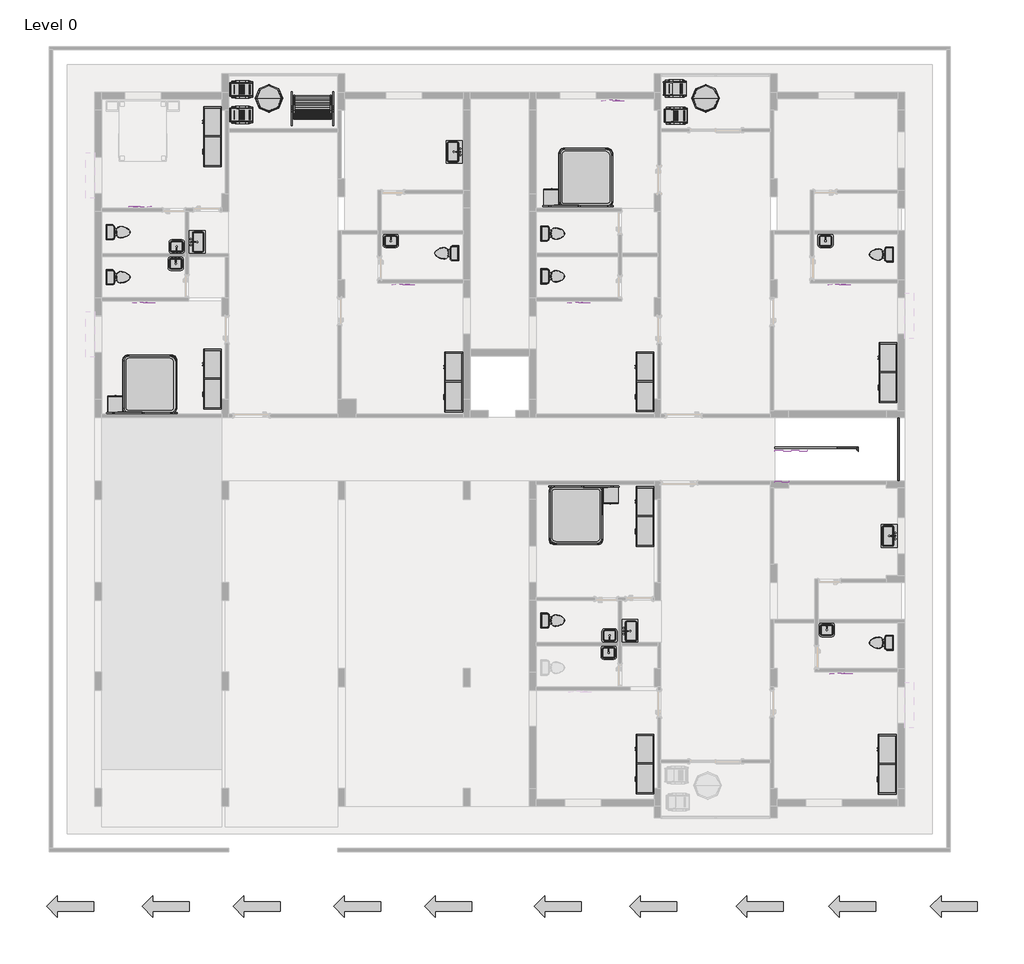
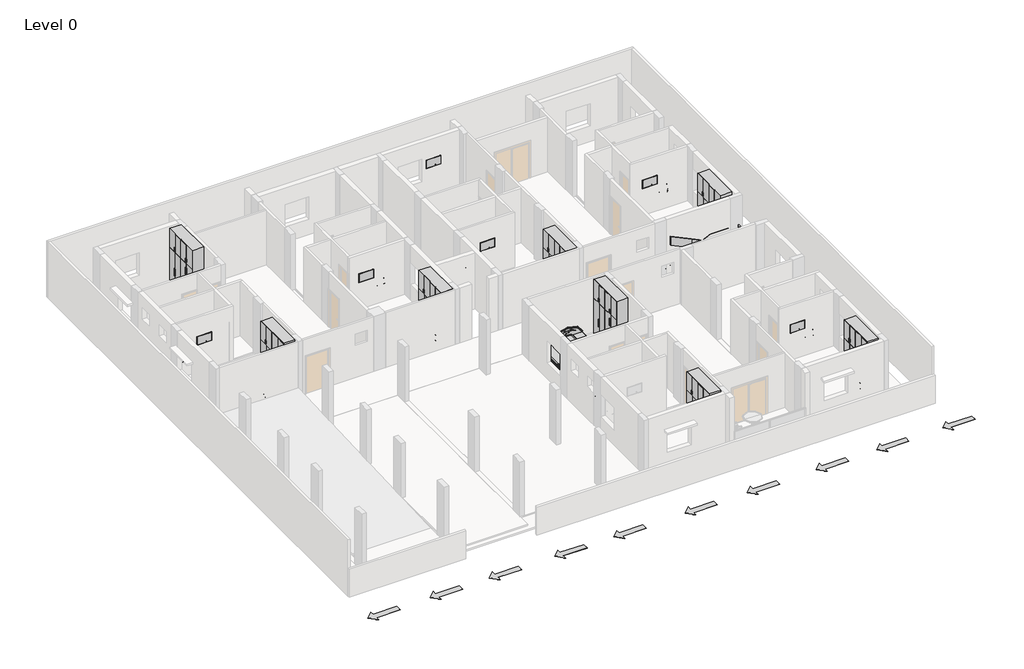
# One storey, part 6 of 6: 19 flow terminals, 18 furniture elements, 10 geographic elements, 8 members, 7 proxies.
"""IFC4 building model written with IfcOpenShell, lengths in millimetres."""

from ifc_helpers import new_model, si_unit, point, frame, frame_2d, origin, place, context, project, spatial, polyline, circle_curve, trimmed, segment, composite_curve, outline, extrude, transform, mapped, element, save
from components import proxy_caca515e, proxy_88c96ab6, flow_terminal_4d548711, flow_terminal_8d9ea526, toilet_domestic_3d_toilet_domestic_3d_ba6479b0, toilet_domestic_3d_toilet_domestic_3d_30431060, furniture_0610_x_0160mm_a8fad5e2, furniture_1wardrobe_6271_1wardrobe_6271_4dd35231, bed_design_8999_bed_design_8999_9c973422, bed_design_8999_bed_design_8999_e911dec7, furniture_f9efd34a, adjustable_garden_chair_5339_adjustable_garden_chair_5339_e938936b, direction_arrows_straight_direction_arrow_straight_a0d3235c

model = new_model("IFC4")

# Units and contexts
model_context = context("Model", 3, world=origin())
ifc_project = project(units=[si_unit("LENGTHUNIT", "METRE", prefix="MILLI")], contexts=[model_context])

# Site, building, storey
site = spatial("IfcSite", under=ifc_project)
building = spatial("IfcBuilding", under=site)
storey = spatial("IfcBuildingStorey", under=building, Name="Level 0", Elevation=0.0)

# Proxies
placement = place(None, origin())
proxy_shape = proxy_caca515e(model_context)
element("IfcBuildingElementProxy", 1, Name="32\" ES6305U", ObjectType="32\" ES6305U", at=placement, inside=storey, context=model_context, shape_type="MappedRepresentation", body=[
    mapped(proxy_shape, transform((-11724.9799383, 3422.4522446, 0.0), x_axis=(-1.0, 0.0, 0.0), y_axis=(0.0, -1.0, 0.0), z_axis=(0.0, 0.0, 1.0))),
])
element("IfcBuildingElementProxy", 2, Name="32\" ES6305U", ObjectType="32\" ES6305U", at=placement, inside=storey, context=model_context, shape_type="MappedRepresentation", body=[
    mapped(proxy_shape, transform((-12079.4641734, 6419.6522446, 0.0), x_axis=(1.0, 0.0, 0.0), y_axis=(0.0, 1.0, 0.0), z_axis=(0.0, 0.0, 1.0))),
])
element("IfcBuildingElementProxy", 3, Name="32\" ES6305U", ObjectType="32\" ES6305U", at=placement, inside=storey, context=model_context, shape_type="MappedRepresentation", body=[
    mapped(proxy_shape, transform((-3047.4141734, 4032.0522446, 0.0), x_axis=(-1.0, 0.0, 0.0), y_axis=(0.0, -1.0, 0.0), z_axis=(0.0, 0.0, 1.0))),
])
element("IfcBuildingElementProxy", 4, Name="32\" ES6305U", ObjectType="32\" ES6305U", at=placement, inside=storey, context=model_context, shape_type="MappedRepresentation", body=[
    mapped(proxy_shape, transform((2839.1098461, 3423.5982139, 0.0), x_axis=(-1.0, 0.0, 0.0), y_axis=(0.0, -1.0, 0.0), z_axis=(0.0, 0.0, 1.0))),
])
element("IfcBuildingElementProxy", 5, Name="32\" ES6305U", ObjectType="32\" ES6305U", at=placement, inside=storey, context=model_context, shape_type="MappedRepresentation", body=[
    mapped(proxy_shape, transform((11538.9418363, 4033.1982139, 0.0), x_axis=(-1.0, 0.0, 0.0), y_axis=(0.0, -1.0, 0.0), z_axis=(0.0, 0.0, 1.0))),
])
element("IfcBuildingElementProxy", 6, Name="32\" ES6305U", ObjectType="32\" ES6305U", at=placement, inside=storey, context=model_context, shape_type="MappedRepresentation", body=[
    mapped(proxy_shape, transform((11614.7358266, -8984.3017861, 0.0), x_axis=(-1.0, 0.0, 0.0), y_axis=(0.0, -1.0, 0.0), z_axis=(0.0, 0.0, 1.0))),
])
proxy_2_shape = proxy_88c96ab6(model_context)
element("IfcBuildingElementProxy", 7, Name="32\" ES6305U", ObjectType="32\" ES6305U", at=placement, inside=storey, context=model_context, shape_type="MappedRepresentation", body=[
    mapped(proxy_2_shape, transform((3975.6858266, 10248.7022446, 0.0), x_axis=(-1.0, 0.0, 0.0), y_axis=(0.0, -1.0, 0.0), z_axis=(0.0, 0.0, 1.0))),
])

# Flow terminals
flow_terminal_shape = flow_terminal_4d548711(model_context)
element("IfcFlowTerminal", 8, ObjectType="Sink Kitchen-Single : 30\" x 21\"", at=placement, inside=storey, context=model_context, shape_type="MappedRepresentation", body=[
    mapped(flow_terminal_shape, transform((-10053.3947528, 5328.8974712, 0.0), x_axis=(0.0, 1.0, 0.0), y_axis=(-1.0, 0.0, 0.0), z_axis=(0.0, 0.0, 1.0))),
])
element("IfcFlowTerminal", 9, ObjectType="Sink Kitchen-Single : 30\" x 21\"", at=placement, inside=storey, context=model_context, shape_type="MappedRepresentation", body=[
    mapped(flow_terminal_shape, transform((-1464.9999296, 8378.8676725, 0.0), x_axis=(0.0, -1.0, 0.0), y_axis=(1.0, 0.0, 0.0), z_axis=(0.0, 0.0, 1.0))),
])
element("IfcFlowTerminal", 10, ObjectType="Sink Kitchen-Single : 30\" x 21\"", at=placement, inside=storey, context=model_context, shape_type="MappedRepresentation", body=[
    mapped(flow_terminal_shape, transform((13087.512135, -4473.7684387, 0.0), x_axis=(0.0, -1.0, 0.0), y_axis=(1.0, 0.0, 0.0), z_axis=(0.0, 0.0, 1.0))),
])
element("IfcFlowTerminal", 11, ObjectType="Sink Kitchen-Single : 30\" x 21\"", at=placement, inside=storey, context=model_context, shape_type="MappedRepresentation", body=[
    mapped(flow_terminal_shape, transform((4424.6052472, -7686.3105902, 0.0), x_axis=(0.0, 1.0, 0.0), y_axis=(-1.0, 0.0, 0.0), z_axis=(0.0, 0.0, 1.0))),
])
flow_terminal_2_shape = flow_terminal_8d9ea526(model_context)
element("IfcFlowTerminal", 12, ObjectType="Sink Vanity-Square : 20\" x 18\"", at=placement, inside=storey, context=model_context, shape_type="MappedRepresentation", body=[
    mapped(flow_terminal_2_shape, transform((-10723.7049515, 5145.6476457, 0.0), x_axis=(-1.0, 0.0, 0.0), y_axis=(0.0, -1.0, 0.0), z_axis=(0.0, 0.0, 1.0))),
])
element("IfcFlowTerminal", 13, ObjectType="Sink Vanity-Square : 20\" x 18\"", at=placement, inside=storey, context=model_context, shape_type="MappedRepresentation", body=[
    mapped(flow_terminal_2_shape, transform((-10785.2606859, 4671.0568434, 0.0), x_axis=(1.0, 0.0, 0.0), y_axis=(0.0, 1.0, 0.0), z_axis=(0.0, 0.0, 1.0))),
])
element("IfcFlowTerminal", 14, ObjectType="Sink Vanity-Square : 20\" x 18\"", at=placement, inside=storey, context=model_context, shape_type="MappedRepresentation", body=[
    mapped(flow_terminal_2_shape, transform((-3592.2834435, 5433.0568435, 0.0), x_axis=(1.0, 0.0, 0.0), y_axis=(0.0, 1.0, 0.0), z_axis=(0.0, 0.0, 1.0))),
])
element("IfcFlowTerminal", 15, ObjectType="Sink Vanity-Square : 20\" x 18\"", at=placement, inside=storey, context=model_context, shape_type="MappedRepresentation", body=[
    mapped(flow_terminal_2_shape, transform((3692.7393144, -8345.2971873, 0.0), x_axis=(1.0, 0.0, 0.0), y_axis=(0.0, 1.0, 0.0), z_axis=(0.0, 0.0, 1.0))),
])
element("IfcFlowTerminal", 16, ObjectType="Sink Vanity-Square : 20\" x 18\"", at=placement, inside=storey, context=model_context, shape_type="MappedRepresentation", body=[
    mapped(flow_terminal_2_shape, transform((3754.2950489, -7870.706385, 0.0), x_axis=(-1.0, 0.0, 0.0), y_axis=(0.0, -1.0, 0.0), z_axis=(0.0, 0.0, 1.0))),
])
element("IfcFlowTerminal", 17, ObjectType="Sink Vanity-Square : 20\" x 18\"", at=placement, inside=storey, context=model_context, shape_type="MappedRepresentation", body=[
    mapped(flow_terminal_2_shape, transform((10988.8893035, -7583.2971873, 0.0), x_axis=(1.0, 0.0, 0.0), y_axis=(0.0, 1.0, 0.0), z_axis=(0.0, 0.0, 1.0))),
])
element("IfcFlowTerminal", 18, ObjectType="Sink Vanity-Square : 20\" x 18\"", at=placement, inside=storey, context=model_context, shape_type="MappedRepresentation", body=[
    mapped(flow_terminal_2_shape, transform((10944.7846056, 5434.2028128, 0.0), x_axis=(1.0, 0.0, 0.0), y_axis=(0.0, 1.0, 0.0), z_axis=(0.0, 0.0, 1.0))),
])
toilet_domestic_3d_toilet_domestic_3d_shape = toilet_domestic_3d_toilet_domestic_3d_ba6479b0(model_context)
toilet_domestic_3d_toilet_domestic_3d_2_shape = toilet_domestic_3d_toilet_domestic_3d_30431060(model_context)
element("IfcFlowTerminal", 19, ObjectType="Toilet-Domestic-3D : Toilet-Domestic-3D", at=placement, inside=storey, context=model_context, shape_type="MappedRepresentation", body=[
    mapped(toilet_domestic_3d_toilet_domestic_3d_shape, transform((-12602.2263533, 5674.4006853, 0.0), x_axis=(0.0, 1.0, 0.0), y_axis=(-1.0, 0.0, 0.0), z_axis=(0.0, 0.0, 1.0))),
    mapped(toilet_domestic_3d_toilet_domestic_3d_2_shape, transform((-12602.2263533, 5674.4006853, 0.0), x_axis=(0.0, 1.0, 0.0), y_axis=(-1.0, 0.0, 0.0), z_axis=(0.0, 0.0, 1.0))),
])
element("IfcFlowTerminal", 20, ObjectType="Toilet-Domestic-3D : Toilet-Domestic-3D", at=placement, inside=storey, context=model_context, shape_type="MappedRepresentation", body=[
    mapped(toilet_domestic_3d_toilet_domestic_3d_shape, transform((-12602.2263533, 4167.1052558, 0.0), x_axis=(0.0, 1.0, 0.0), y_axis=(-1.0, 0.0, 0.0), z_axis=(0.0, 0.0, 1.0))),
    mapped(toilet_domestic_3d_toilet_domestic_3d_2_shape, transform((-12602.2263533, 4167.1052558, 0.0), x_axis=(0.0, 1.0, 0.0), y_axis=(-1.0, 0.0, 0.0), z_axis=(0.0, 0.0, 1.0))),
])
element("IfcFlowTerminal", 21, ObjectType="Toilet-Domestic-3D : Toilet-Domestic-3D", at=placement, inside=storey, context=model_context, shape_type="MappedRepresentation", body=[
    mapped(toilet_domestic_3d_toilet_domestic_3d_shape, transform((1932.9236467, 5629.7891838, 0.0), x_axis=(0.0, 1.0, 0.0), y_axis=(-1.0, 0.0, 0.0), z_axis=(0.0, 0.0, 1.0))),
    mapped(toilet_domestic_3d_toilet_domestic_3d_2_shape, transform((1932.9236467, 5629.7891838, 0.0), x_axis=(0.0, 1.0, 0.0), y_axis=(-1.0, 0.0, 0.0), z_axis=(0.0, 0.0, 1.0))),
])
element("IfcFlowTerminal", 22, ObjectType="Toilet-Domestic-3D : Toilet-Domestic-3D", at=placement, inside=storey, context=model_context, shape_type="MappedRepresentation", body=[
    mapped(toilet_domestic_3d_toilet_domestic_3d_shape, transform((1932.9236467, 4198.8992096, 0.0), x_axis=(0.0, 1.0, 0.0), y_axis=(-1.0, 0.0, 0.0), z_axis=(0.0, 0.0, 1.0))),
    mapped(toilet_domestic_3d_toilet_domestic_3d_2_shape, transform((1932.9236467, 4198.8992096, 0.0), x_axis=(0.0, 1.0, 0.0), y_axis=(-1.0, 0.0, 0.0), z_axis=(0.0, 0.0, 1.0))),
])
element("IfcFlowTerminal", 23, ObjectType="Toilet-Domestic-3D : Toilet-Domestic-3D", at=placement, inside=storey, context=model_context, shape_type="MappedRepresentation", body=[
    mapped(toilet_domestic_3d_toilet_domestic_3d_shape, transform((12734.5531459, 4928.5482139, 0.0), x_axis=(0.0, -1.0, 0.0), y_axis=(1.0, 0.0, 0.0), z_axis=(0.0, 0.0, 1.0))),
    mapped(toilet_domestic_3d_toilet_domestic_3d_2_shape, transform((12734.5531459, 4928.5482139, 0.0), x_axis=(0.0, -1.0, 0.0), y_axis=(1.0, 0.0, 0.0), z_axis=(0.0, 0.0, 1.0))),
])
element("IfcFlowTerminal", 24, ObjectType="Toilet-Domestic-3D : Toilet-Domestic-3D", at=placement, inside=storey, context=model_context, shape_type="MappedRepresentation", body=[
    mapped(toilet_domestic_3d_toilet_domestic_3d_shape, transform((12734.5531459, -8063.5517861, 0.0), x_axis=(0.0, -1.0, 0.0), y_axis=(1.0, 0.0, 0.0), z_axis=(0.0, 0.0, 1.0))),
    mapped(toilet_domestic_3d_toilet_domestic_3d_2_shape, transform((12734.5531459, -8063.5517861, 0.0), x_axis=(0.0, -1.0, 0.0), y_axis=(1.0, 0.0, 0.0), z_axis=(0.0, 0.0, 1.0))),
])
element("IfcFlowTerminal", 25, ObjectType="Toilet-Domestic-3D : Toilet-Domestic-3D", at=placement, inside=storey, context=model_context, shape_type="MappedRepresentation", body=[
    mapped(toilet_domestic_3d_toilet_domestic_3d_shape, transform((1932.9236467, -7320.9899443, 0.0), x_axis=(0.0, 1.0, 0.0), y_axis=(-1.0, 0.0, 0.0), z_axis=(0.0, 0.0, 1.0))),
    mapped(toilet_domestic_3d_toilet_domestic_3d_2_shape, transform((1932.9236467, -7320.9899443, 0.0), x_axis=(0.0, 1.0, 0.0), y_axis=(-1.0, 0.0, 0.0), z_axis=(0.0, 0.0, 1.0))),
])
element("IfcFlowTerminal", 26, ObjectType="Toilet-Domestic-3D : Toilet-Domestic-3D", at=placement, inside=storey, context=model_context, shape_type="MappedRepresentation", body=[
    mapped(toilet_domestic_3d_toilet_domestic_3d_shape, transform((-1800.5968541, 4969.1674323, 0.0), x_axis=(0.0, -1.0, 0.0), y_axis=(1.0, 0.0, 0.0), z_axis=(0.0, 0.0, 1.0))),
    mapped(toilet_domestic_3d_toilet_domestic_3d_2_shape, transform((-1800.5968541, 4969.1674323, 0.0), x_axis=(0.0, -1.0, 0.0), y_axis=(1.0, 0.0, 0.0), z_axis=(0.0, 0.0, 1.0))),
])

# Furniture
furniture_0610_x_0160mm_shape = furniture_0610_x_0160mm_a8fad5e2(model_context)
element("IfcFurniture", 27, ObjectType="0610 x 0160mm", at=placement, inside=storey, context=model_context, shape_type="MappedRepresentation", body=[
    mapped(furniture_0610_x_0160mm_shape, transform((-5755.1495977, 10726.8303324, 0.0), x_axis=(-1.0, 0.0, 0.0), y_axis=(0.0, -1.0, 0.0), z_axis=(0.0, 0.0, 1.0))),
])
element("IfcFurniture", 28, ObjectType="1Wardrobe_6271 : 1Wardrobe_6271", at=placement, inside=storey, context=model_context, shape_type="SweptSolid", body=[
    extrude(outline(polyline([(-9841.4902865, 7867.8575257), (-9841.4902865, 8857.8575257), (-9821.4902865, 8857.8575257), (-9821.4902865, 7867.8575257), (-9841.4902865, 7867.8575257)])), frame((0.0, 0.0, 532.0), z_axis=(0.0, 0.0, 1.0), x_axis=(1.0, 0.0, 0.0)), (0.0, 0.0, 1.0), 285.0),
    extrude(outline(composite_curve([segment(trimmed(circle_curve(frame_2d((272.2650104, -9866.4893345)), 7.5), [point((264.7650104, -9866.4893345))], [point((279.7650104, -9866.4893345))], False, "CARTESIAN"), True, "CONTINUOUS"), segment(trimmed(circle_curve(frame_2d((272.2650104, -9866.4893345)), 7.5), [point((279.7650104, -9866.4893345))], [point((264.7650104, -9866.4893345))], False, "CARTESIAN"), True, "CONTINUOUS")], self_intersect=False)), frame((0.0, 8285.9077329, 0.0), z_axis=(0.0, 1.0, 0.0), x_axis=(0.0, 0.0, 1.0)), (0.0, 0.0, 1.0), 160.0),
    extrude(outline(composite_curve([segment(trimmed(circle_curve(frame_2d((577.2650104, -9866.4893345)), 7.5), [point((569.7650104, -9866.4893345))], [point((584.7650104, -9866.4893345))], False, "CARTESIAN"), True, "CONTINUOUS"), segment(trimmed(circle_curve(frame_2d((577.2650104, -9866.4893345)), 7.5), [point((584.7650104, -9866.4893345))], [point((569.7650104, -9866.4893345))], False, "CARTESIAN"), True, "CONTINUOUS")], self_intersect=False)), frame((0.0, 8285.9077329, 0.0), z_axis=(0.0, 1.0, 0.0), x_axis=(0.0, 0.0, 1.0)), (0.0, 0.0, 1.0), 160.0),
    extrude(outline(polyline([(-9841.4902865, 7867.8575257), (-9841.4902865, 8357.8575257), (-9821.4902865, 8357.8575257), (-9821.4902865, 7867.8575257), (-9841.4902865, 7867.8575257)])), frame((0.0, 0.0, 2137.0), z_axis=(0.0, 0.0, 1.0), x_axis=(1.0, 0.0, 0.0)), (0.0, 0.0, 1.0), 990.0),
    extrude(outline(composite_curve([segment(trimmed(circle_curve(frame_2d((-9866.4893345, 9327.8010612)), 7.5), [point((-9866.4893345, 9320.3010612))], [point((-9866.4893345, 9335.3010612))], False, "CARTESIAN"), True, "CONTINUOUS"), segment(trimmed(circle_curve(frame_2d((-9866.4893345, 9327.8010612)), 7.5), [point((-9866.4893345, 9335.3010612))], [point((-9866.4893345, 9320.3010612))], False, "CARTESIAN"), True, "CONTINUOUS")], self_intersect=False)), frame((0.0, 0.0, 2237.0), z_axis=(0.0, 0.0, 1.0), x_axis=(1.0, 0.0, 0.0)), (0.0, 0.0, 1.0), 160.0),
    extrude(outline(composite_curve([segment(trimmed(circle_curve(frame_2d((-9866.4893345, 9407.9139903)), 7.5), [point((-9866.4893345, 9415.4139903))], [point((-9866.4893345, 9400.4139903))], False, "CARTESIAN"), True, "CONTINUOUS"), segment(trimmed(circle_curve(frame_2d((-9866.4893345, 9407.9139903)), 7.5), [point((-9866.4893345, 9400.4139903))], [point((-9866.4893345, 9415.4139903))], False, "CARTESIAN"), True, "CONTINUOUS")], self_intersect=False)), frame((0.0, 0.0, 2237.0), z_axis=(0.0, 0.0, 1.0), x_axis=(1.0, 0.0, 0.0)), (0.0, 0.0, 1.0), 160.0),
    extrude(outline(composite_curve([segment(trimmed(circle_curve(frame_2d((-9866.4893345, 8407.9139903)), 7.5), [point((-9866.4893345, 8415.4139903))], [point((-9866.4893345, 8400.4139903))], False, "CARTESIAN"), True, "CONTINUOUS"), segment(trimmed(circle_curve(frame_2d((-9866.4893345, 8407.9139903)), 7.5), [point((-9866.4893345, 8400.4139903))], [point((-9866.4893345, 8415.4139903))], False, "CARTESIAN"), True, "CONTINUOUS")], self_intersect=False)), frame((0.0, 0.0, 2237.0), z_axis=(0.0, 0.0, 1.0), x_axis=(1.0, 0.0, 0.0)), (0.0, 0.0, 1.0), 160.0),
    extrude(outline(composite_curve([segment(trimmed(circle_curve(frame_2d((-9866.4893345, 8327.8010612)), 7.5), [point((-9866.4893345, 8320.3010612))], [point((-9866.4893345, 8335.3010612))], False, "CARTESIAN"), True, "CONTINUOUS"), segment(trimmed(circle_curve(frame_2d((-9866.4893345, 8327.8010612)), 7.5), [point((-9866.4893345, 8335.3010612))], [point((-9866.4893345, 8320.3010612))], False, "CARTESIAN"), True, "CONTINUOUS")], self_intersect=False)), frame((0.0, 0.0, 2237.0), z_axis=(0.0, 0.0, 1.0), x_axis=(1.0, 0.0, 0.0)), (0.0, 0.0, 1.0), 160.0),
    extrude(outline(polyline([(-9841.4902865, 8367.8575257), (-9841.4902865, 8857.8575257), (-9821.4902865, 8857.8575257), (-9821.4902865, 8367.8575257), (-9841.4902865, 8367.8575257)])), frame((0.0, 0.0, 2137.0), z_axis=(0.0, 0.0, 1.0), x_axis=(1.0, 0.0, 0.0)), (0.0, 0.0, 1.0), 990.0),
    extrude(outline(polyline([(-9841.4902865, 8367.8575257), (-9841.4902865, 8857.8575257), (-9821.4902865, 8857.8575257), (-9821.4902865, 8367.8575257), (-9841.4902865, 8367.8575257)])), frame((0.0, 0.0, 832.0), z_axis=(0.0, 0.0, 1.0), x_axis=(1.0, 0.0, 0.0)), (0.0, 0.0, 1.0), 1285.0),
    extrude(outline(polyline([(-9841.4902865, 7867.8575257), (-9841.4902865, 8357.8575257), (-9821.4902865, 8357.8575257), (-9821.4902865, 7867.8575257), (-9841.4902865, 7867.8575257)])), frame((0.0, 0.0, 832.0), z_axis=(0.0, 0.0, 1.0), x_axis=(1.0, 0.0, 0.0)), (0.0, 0.0, 1.0), 1285.0),
    extrude(outline(polyline([(-9841.4902865, 8877.8575257), (-9841.4902865, 9367.8575257), (-9821.4902865, 9367.8575257), (-9821.4902865, 8877.8575257), (-9841.4902865, 8877.8575257)])), frame((0.0, 0.0, 227.0), z_axis=(0.0, 0.0, 1.0), x_axis=(1.0, 0.0, 0.0)), (0.0, 0.0, 1.0), 1890.0),
    extrude(outline(polyline([(-9841.4902865, 9377.8575257), (-9841.4902865, 9867.8575257), (-9821.4902865, 9867.8575257), (-9821.4902865, 9377.8575257), (-9841.4902865, 9377.8575257)])), frame((0.0, 0.0, 2137.0), z_axis=(0.0, 0.0, 1.0), x_axis=(1.0, 0.0, 0.0)), (0.0, 0.0, 1.0), 990.0),
    extrude(outline(composite_curve([segment(trimmed(circle_curve(frame_2d((-9866.4902865, 8327.8575257)), 10.0), [point((-9866.4902865, 8337.8575257))], [point((-9866.4902865, 8317.8575257))], False, "CARTESIAN"), True, "CONTINUOUS"), segment(trimmed(circle_curve(frame_2d((-9866.4902865, 8327.8575257)), 10.0), [point((-9866.4902865, 8317.8575257))], [point((-9866.4902865, 8337.8575257))], False, "CARTESIAN"), True, "CONTINUOUS")], self_intersect=False)), frame((0.0, 0.0, 1537.0), z_axis=(0.0, 0.0, 1.0), x_axis=(1.0, 0.0, 0.0)), (0.0, 0.0, 1.0), 380.0),
    extrude(outline(composite_curve([segment(trimmed(circle_curve(frame_2d((-9866.4902865, 8407.8575257)), 10.0), [point((-9866.4902865, 8397.8575257))], [point((-9866.4902865, 8417.8575257))], False, "CARTESIAN"), True, "CONTINUOUS"), segment(trimmed(circle_curve(frame_2d((-9866.4902865, 8407.8575257)), 10.0), [point((-9866.4902865, 8417.8575257))], [point((-9866.4902865, 8397.8575257))], False, "CARTESIAN"), True, "CONTINUOUS")], self_intersect=False)), frame((0.0, 0.0, 1537.0), z_axis=(0.0, 0.0, 1.0), x_axis=(1.0, 0.0, 0.0)), (0.0, 0.0, 1.0), 380.0),
    extrude(outline(composite_curve([segment(trimmed(circle_curve(frame_2d((-9866.4902865, 9327.8575257)), 10.0), [point((-9866.4902865, 9337.8575257))], [point((-9866.4902865, 9317.8575257))], False, "CARTESIAN"), True, "CONTINUOUS"), segment(trimmed(circle_curve(frame_2d((-9866.4902865, 9327.8575257)), 10.0), [point((-9866.4902865, 9317.8575257))], [point((-9866.4902865, 9337.8575257))], False, "CARTESIAN"), True, "CONTINUOUS")], self_intersect=False)), frame((0.0, 0.0, 860.2017452), z_axis=(0.0, 0.0, 1.0), x_axis=(1.0, 0.0, 0.0)), (0.0, 0.0, 1.0), 380.0),
    extrude(outline(composite_curve([segment(trimmed(circle_curve(frame_2d((-9866.4902865, 9407.8575257)), 10.0), [point((-9866.4902865, 9397.8575257))], [point((-9866.4902865, 9417.8575257))], False, "CARTESIAN"), True, "CONTINUOUS"), segment(trimmed(circle_curve(frame_2d((-9866.4902865, 9407.8575257)), 10.0), [point((-9866.4902865, 9417.8575257))], [point((-9866.4902865, 9397.8575257))], False, "CARTESIAN"), True, "CONTINUOUS")], self_intersect=False)), frame((0.0, 0.0, 860.2017452), z_axis=(0.0, 0.0, 1.0), x_axis=(1.0, 0.0, 0.0)), (0.0, 0.0, 1.0), 380.0),
    extrude(outline(polyline([(-9821.4902865, 8867.8575257), (-9821.4902865, 9827.8575257), (-9261.4902865, 9827.8575257), (-9261.4902865, 8867.8575257), (-9821.4902865, 8867.8575257)])), frame((0.0, 0.0, 2107.0), z_axis=(0.0, 0.0, 1.0), x_axis=(1.0, 0.0, 0.0)), (0.0, 0.0, 1.0), 40.0),
    extrude(outline(polyline([(-9821.4902865, 7907.8575257), (-9821.4902865, 8917.8575257), (-9261.4902865, 8917.8575257), (-9261.4902865, 7907.8575257), (-9821.4902865, 7907.8575257)])), frame((0.0, 0.0, 2107.0), z_axis=(0.0, 0.0, 1.0), x_axis=(1.0, 0.0, 0.0)), (0.0, 0.0, 1.0), 40.0),
    extrude(outline(polyline([(-9821.4902865, 8907.8575257), (-9821.4902865, 9827.8575257), (-9261.4902865, 9827.8575257), (-9261.4902865, 8907.8575257), (-9821.4902865, 8907.8575257)])), frame((0.0, 0.0, 2627.0), z_axis=(0.0, 0.0, 1.0), x_axis=(1.0, 0.0, 0.0)), (0.0, 0.0, 1.0), 40.0),
    extrude(outline(polyline([(-9821.4902865, 8867.8575257), (-9821.4902865, 8907.8575257), (-9261.4902865, 8907.8575257), (-9261.4902865, 8867.8575257), (-9821.4902865, 8867.8575257)])), frame((0.0, 0.0, 227.0), z_axis=(0.0, 0.0, 1.0), x_axis=(1.0, 0.0, 0.0)), (0.0, 0.0, 1.0), 2860.0),
    extrude(outline(polyline([(-9261.4902865, 7907.8575257), (-9261.4902865, 9827.8575257), (-9241.4902865, 9827.8575257), (-9241.4902865, 7907.8575257), (-9261.4902865, 7907.8575257)])), frame((0.0, 0.0, 227.0), z_axis=(0.0, 0.0, 1.0), x_axis=(1.0, 0.0, 0.0)), (0.0, 0.0, 1.0), 2860.0),
    extrude(outline(polyline([(9867.8575257, 3127.0), (9867.8575257, 227.0), (9827.8575257, 227.0), (9827.8575257, 3087.0), (7907.8575257, 3087.0), (7907.8575257, 227.0), (7867.8575257, 227.0), (7867.8575257, 3127.0), (9867.8575257, 3127.0)])), frame((-9821.4902865, 0.0, 0.0), z_axis=(1.0, 0.0, 0.0), x_axis=(0.0, 1.0, 0.0)), (0.0, 0.0, 1.0), 580.0),
    extrude(outline(polyline([(-9841.4902865, 7867.8575257), (-9841.4902865, 8857.8575257), (-9821.4902865, 8857.8575257), (-9821.4902865, 7867.8575257), (-9841.4902865, 7867.8575257)])), frame((0.0, 0.0, 227.0), z_axis=(0.0, 0.0, 1.0), x_axis=(1.0, 0.0, 0.0)), (0.0, 0.0, 1.0), 285.0),
    extrude(outline(polyline([(-9841.4902865, 8877.8575257), (-9841.4902865, 9367.8575257), (-9821.4902865, 9367.8575257), (-9821.4902865, 8877.8575257), (-9841.4902865, 8877.8575257)])), frame((0.0, 0.0, 2137.0), z_axis=(0.0, 0.0, 1.0), x_axis=(1.0, 0.0, 0.0)), (0.0, 0.0, 1.0), 990.0),
    extrude(outline(polyline([(-9841.4902865, 9377.8575257), (-9841.4902865, 9867.8575257), (-9821.4902865, 9867.8575257), (-9821.4902865, 9377.8575257), (-9841.4902865, 9377.8575257)])), frame((0.0, 0.0, 227.0), z_axis=(0.0, 0.0, 1.0), x_axis=(1.0, 0.0, 0.0)), (0.0, 0.0, 1.0), 1890.0),
    extrude(outline(polyline([(-9841.4902865, 7867.8575257), (-9841.4902865, 9867.8575257), (-9241.4902865, 9867.8575257), (-9241.4902865, 7867.8575257), (-9841.4902865, 7867.8575257)])), frame((0.0, 0.0, 127.0), z_axis=(0.0, 0.0, 1.0), x_axis=(1.0, 0.0, 0.0)), (0.0, 0.0, 1.0), 100.0),
])
furniture_1wardrobe_6271_1wardrobe_6271_shape = furniture_1wardrobe_6271_1wardrobe_6271_4dd35231(model_context)
element("IfcFurniture", 29, ObjectType="1Wardrobe_6271 : 1Wardrobe_6271", at=placement, inside=storey, context=model_context, shape_type="MappedRepresentation", body=[
    mapped(furniture_1wardrobe_6271_1wardrobe_6271_shape, transform((-1178.4401539, 1664.6482139, 0.0), x_axis=(0.0, -1.0, 0.0), y_axis=(1.0, 0.0, 0.0), z_axis=(0.0, 0.0, 1.0))),
])
element("IfcFurniture", 30, ObjectType="1Wardrobe_6271 : 1Wardrobe_6271", at=placement, inside=storey, context=model_context, shape_type="MappedRepresentation", body=[
    mapped(furniture_1wardrobe_6271_1wardrobe_6271_shape, transform((-9241.4902865, 1755.675995, 0.0), x_axis=(0.0, -1.0, 0.0), y_axis=(1.0, 0.0, 0.0), z_axis=(0.0, 0.0, 1.0))),
])
element("IfcFurniture", 31, ObjectType="1Wardrobe_6271 : 1Wardrobe_6271", at=placement, inside=storey, context=model_context, shape_type="MappedRepresentation", body=[
    mapped(furniture_1wardrobe_6271_1wardrobe_6271_shape, transform((13352.5198768, 1974.4442547, 0.0), x_axis=(0.0, -1.0, 0.0), y_axis=(1.0, 0.0, 0.0), z_axis=(0.0, 0.0, 1.0))),
])
element("IfcFurniture", 32, ObjectType="1Wardrobe_6271 : 1Wardrobe_6271", at=placement, inside=storey, context=model_context, shape_type="MappedRepresentation", body=[
    mapped(furniture_1wardrobe_6271_1wardrobe_6271_shape, transform((5224.5198768, 1666.9822153, 0.0), x_axis=(0.0, -1.0, 0.0), y_axis=(1.0, 0.0, 0.0), z_axis=(0.0, 0.0, 1.0))),
])
element("IfcFurniture", 33, ObjectType="1Wardrobe_6271 : 1Wardrobe_6271", at=placement, inside=storey, context=model_context, shape_type="MappedRepresentation", body=[
    mapped(furniture_1wardrobe_6271_1wardrobe_6271_shape, transform((5225.3507059, -2841.9517861, 0.0), x_axis=(0.0, -1.0, 0.0), y_axis=(1.0, 0.0, 0.0), z_axis=(0.0, 0.0, 1.0))),
])
element("IfcFurniture", 34, ObjectType="1Wardrobe_6271 : 1Wardrobe_6271", at=placement, inside=storey, context=model_context, shape_type="MappedRepresentation", body=[
    mapped(furniture_1wardrobe_6271_1wardrobe_6271_shape, transform((5225.3507059, -11122.3517861, 0.0), x_axis=(0.0, -1.0, 0.0), y_axis=(1.0, 0.0, 0.0), z_axis=(0.0, 0.0, 1.0))),
])
element("IfcFurniture", 35, ObjectType="1Wardrobe_6271 : 1Wardrobe_6271", at=placement, inside=storey, context=model_context, shape_type="MappedRepresentation", body=[
    mapped(furniture_1wardrobe_6271_1wardrobe_6271_shape, transform((13326.7205092, -11133.7852089, 0.0), x_axis=(0.0, -1.0, 0.0), y_axis=(1.0, 0.0, 0.0), z_axis=(0.0, 0.0, 1.0))),
])
bed_design_8999_bed_design_8999_shape = bed_design_8999_bed_design_8999_9c973422(model_context)
bed_design_8999_bed_design_8999_2_shape = bed_design_8999_bed_design_8999_e911dec7(model_context)
element("IfcFurniture", 36, ObjectType="BED_DESIGN_8999 : BED_DESIGN_8999", at=placement, inside=storey, context=model_context, shape_type="MappedRepresentation", body=[
    mapped(bed_design_8999_bed_design_8999_shape, transform((-11841.3445465, 1563.0482139, 0.0), x_axis=(-0.9999998636386791, -0.0005222285163069755, 0.0), y_axis=(0.0005222285163069755, -0.9999998636386791, 0.0), z_axis=(0.0, 0.0, 1.0))),
    mapped(bed_design_8999_bed_design_8999_2_shape, transform((-11841.3445465, 1563.0482139, 0.0), x_axis=(-0.9999998636386791, -0.0005222285163069755, 0.0), y_axis=(0.0005222285163069755, -0.9999998636386791, 0.0), z_axis=(0.0, 0.0, 1.0))),
])
element("IfcFurniture", 37, ObjectType="BED_DESIGN_8999 : BED_DESIGN_8999", at=placement, inside=storey, context=model_context, shape_type="MappedRepresentation", body=[
    mapped(bed_design_8999_bed_design_8999_shape, transform((2747.6199328, 8482.7740437, 0.0), x_axis=(-0.9999998636386791, -0.0005222285163069755, 0.0), y_axis=(0.0005222285163069755, -0.9999998636386791, 0.0), z_axis=(0.0, 0.0, 1.0))),
    mapped(bed_design_8999_bed_design_8999_2_shape, transform((2747.6199328, 8482.7740437, 0.0), x_axis=(-0.9999998636386791, -0.0005222285163069755, 0.0), y_axis=(0.0005222285163069755, -0.9999998636386791, 0.0), z_axis=(0.0, 0.0, 1.0))),
])
element("IfcFurniture", 38, ObjectType="BED_DESIGN_8999 : BED_DESIGN_8999", at=placement, inside=storey, context=model_context, shape_type="MappedRepresentation", body=[
    mapped(bed_design_8999_bed_design_8999_shape, transform((2819.4944717, -4774.2138445, 0.0), x_axis=(0.9999998636386791, 0.0005222285163058449, 0.0), y_axis=(-0.0005222285163058449, 0.9999998636386791, 0.0), z_axis=(0.0, 0.0, 1.0))),
    mapped(bed_design_8999_bed_design_8999_2_shape, transform((2819.4944717, -4774.2138445, 0.0), x_axis=(0.9999998636386791, 0.0005222285163058449, 0.0), y_axis=(-0.0005222285163058449, 0.9999998636386791, 0.0), z_axis=(0.0, 0.0, 1.0))),
])
furniture_shape = furniture_f9efd34a(model_context)
element("IfcFurniture", 39, ObjectType="Table-Round : 36\" Diameter", at=placement, inside=storey, context=model_context, shape_type="MappedRepresentation", body=[
    mapped(furniture_shape, transform((-7652.6948528, 10153.8482257, 0.0), x_axis=(1.0, 0.0, 0.0), y_axis=(0.0, 1.0, 0.0), z_axis=(0.0, 0.0, 1.0))),
])
element("IfcFurniture", 40, ObjectType="Table-Round : 36\" Diameter", at=placement, inside=storey, context=model_context, shape_type="MappedRepresentation", body=[
    mapped(furniture_shape, transform((6952.3051472, 10153.8482257, 0.0), x_axis=(1.0, 0.0, 0.0), y_axis=(0.0, 1.0, 0.0), z_axis=(0.0, 0.0, 1.0))),
])
adjustable_garden_chair_5339_adjustable_garden_chair_5339_shape = adjustable_garden_chair_5339_adjustable_garden_chair_5339_e938936b(model_context)
element("IfcFurniture", 41, ObjectType="adjustable_garden_chair_5339 : adjustable_garden_chair_5339", at=placement, inside=storey, context=model_context, shape_type="MappedRepresentation", body=[
    mapped(adjustable_garden_chair_5339_adjustable_garden_chair_5339_shape, transform((-8593.324512, 10451.9022446, 0.0), x_axis=(0.0, 1.0, 0.0), y_axis=(-1.0, 0.0, 0.0), z_axis=(0.0, 0.0, 1.0))),
])
element("IfcFurniture", 42, ObjectType="adjustable_garden_chair_5339 : adjustable_garden_chair_5339", at=placement, inside=storey, context=model_context, shape_type="MappedRepresentation", body=[
    mapped(adjustable_garden_chair_5339_adjustable_garden_chair_5339_shape, transform((-8593.324512, 9599.8562752, 0.0), x_axis=(0.0, 1.0, 0.0), y_axis=(-1.0, 0.0, 0.0), z_axis=(0.0, 0.0, 1.0))),
])
element("IfcFurniture", 43, ObjectType="adjustable_garden_chair_5339 : adjustable_garden_chair_5339", at=placement, inside=storey, context=model_context, shape_type="MappedRepresentation", body=[
    mapped(adjustable_garden_chair_5339_adjustable_garden_chair_5339_shape, transform((5914.0489952, 10479.707572, 0.0), x_axis=(0.0, 1.0, 0.0), y_axis=(-1.0, 0.0, 0.0), z_axis=(0.0, 0.0, 1.0))),
])
element("IfcFurniture", 44, ObjectType="adjustable_garden_chair_5339 : adjustable_garden_chair_5339", at=placement, inside=storey, context=model_context, shape_type="MappedRepresentation", body=[
    mapped(adjustable_garden_chair_5339_adjustable_garden_chair_5339_shape, transform((5939.9098461, 9573.6866027, 0.0), x_axis=(0.0, 1.0, 0.0), y_axis=(-1.0, 0.0, 0.0), z_axis=(0.0, 0.0, 1.0))),
])

# Geographic elements
direction_arrows_straight_direction_arrow_straight_shape = direction_arrows_straight_direction_arrow_straight_a0d3235c(model_context)
element("IfcGeographicElement", 45, ObjectType="Direction Arrows - Straight : Direction Arrow - Straight", at=placement, inside=storey, context=model_context, shape_type="MappedRepresentation", body=[
    mapped(direction_arrows_straight_direction_arrow_straight_shape, transform((-13516.4901539, -16890.0517861, 0.0), x_axis=(0.0, 1.0, 0.0), y_axis=(-1.0, 0.0, 0.0), z_axis=(0.0, 0.0, 1.0))),
])
element("IfcGeographicElement", 46, ObjectType="Direction Arrows - Straight : Direction Arrow - Straight", at=placement, inside=storey, context=model_context, shape_type="MappedRepresentation", body=[
    mapped(direction_arrows_straight_direction_arrow_straight_shape, transform((-10316.0901539, -16890.0517861, 0.0), x_axis=(0.0, 1.0, 0.0), y_axis=(-1.0, 0.0, 0.0), z_axis=(0.0, 0.0, 1.0))),
])
element("IfcGeographicElement", 47, ObjectType="Direction Arrows - Straight : Direction Arrow - Straight", at=placement, inside=storey, context=model_context, shape_type="MappedRepresentation", body=[
    mapped(direction_arrows_straight_direction_arrow_straight_shape, transform((-7268.0901539, -16890.0517861, 0.0), x_axis=(0.0, 1.0, 0.0), y_axis=(-1.0, 0.0, 0.0), z_axis=(0.0, 0.0, 1.0))),
])
element("IfcGeographicElement", 48, ObjectType="Direction Arrows - Straight : Direction Arrow - Straight", at=placement, inside=storey, context=model_context, shape_type="MappedRepresentation", body=[
    mapped(direction_arrows_straight_direction_arrow_straight_shape, transform((-3915.2901539, -16890.0517861, 0.0), x_axis=(0.0, 1.0, 0.0), y_axis=(-1.0, 0.0, 0.0), z_axis=(0.0, 0.0, 1.0))),
])
element("IfcGeographicElement", 49, ObjectType="Direction Arrows - Straight : Direction Arrow - Straight", at=placement, inside=storey, context=model_context, shape_type="MappedRepresentation", body=[
    mapped(direction_arrows_straight_direction_arrow_straight_shape, transform((-867.2901539, -16890.0517861, 0.0), x_axis=(0.0, 1.0, 0.0), y_axis=(-1.0, 0.0, 0.0), z_axis=(0.0, 0.0, 1.0))),
])
element("IfcGeographicElement", 50, ObjectType="Direction Arrows - Straight : Direction Arrow - Straight", at=placement, inside=storey, context=model_context, shape_type="MappedRepresentation", body=[
    mapped(direction_arrows_straight_direction_arrow_straight_shape, transform((2790.3098461, -16890.0517861, 0.0), x_axis=(0.0, 1.0, 0.0), y_axis=(-1.0, 0.0, 0.0), z_axis=(0.0, 0.0, 1.0))),
])
element("IfcGeographicElement", 51, ObjectType="Direction Arrows - Straight : Direction Arrow - Straight", at=placement, inside=storey, context=model_context, shape_type="MappedRepresentation", body=[
    mapped(direction_arrows_straight_direction_arrow_straight_shape, transform((5990.7098461, -16890.0517861, 0.0), x_axis=(0.0, 1.0, 0.0), y_axis=(-1.0, 0.0, 0.0), z_axis=(0.0, 0.0, 1.0))),
])
element("IfcGeographicElement", 52, ObjectType="Direction Arrows - Straight : Direction Arrow - Straight", at=placement, inside=storey, context=model_context, shape_type="MappedRepresentation", body=[
    mapped(direction_arrows_straight_direction_arrow_straight_shape, transform((9546.7098461, -16890.0517861, 0.0), x_axis=(0.0, 1.0, 0.0), y_axis=(-1.0, 0.0, 0.0), z_axis=(0.0, 0.0, 1.0))),
])
element("IfcGeographicElement", 53, ObjectType="Direction Arrows - Straight : Direction Arrow - Straight", at=placement, inside=storey, context=model_context, shape_type="MappedRepresentation", body=[
    mapped(direction_arrows_straight_direction_arrow_straight_shape, transform((12640.3587866, -16890.0517861, 0.0), x_axis=(0.0, 1.0, 0.0), y_axis=(-1.0, 0.0, 0.0), z_axis=(0.0, 0.0, 1.0))),
])
element("IfcGeographicElement", 54, ObjectType="Direction Arrows - Straight : Direction Arrow - Straight", at=placement, inside=storey, context=model_context, shape_type="MappedRepresentation", body=[
    mapped(direction_arrows_straight_direction_arrow_straight_shape, transform((16043.9587866, -16890.0517861, 0.0), x_axis=(0.0, 1.0, 0.0), y_axis=(-1.0, 0.0, 0.0), z_axis=(0.0, 0.0, 1.0))),
])

# Members
element("IfcMember", 55, ObjectType="Stringer-50mm_Width", at=placement, inside=storey, context=model_context, shape_type="SweptSolid", body=[
    extrude(outline(polyline([(213.9682309, 9267.2639698), (0.0, 9267.2639698), (0.0, 9748.306958), (1493.8650796, 12885.4236755), (1493.8650796, 11955.0473953), (213.9682309, 9267.2639698)])), frame((0.0, -519.7517861, 0.0), z_axis=(0.0, 1.0, 0.0), x_axis=(0.0, 0.0, 1.0)), (0.0, 0.0, 1.0), 50.0),
])
element("IfcMember", 56, ObjectType="Stringer-50mm_Width", at=placement, inside=storey, context=model_context, shape_type="SweptSolid", body=[
    extrude(outline(polyline([(13382.1098414, -469.7517861), (13432.1098414, -469.7517861), (13432.1098414, -2653.3517861), (13382.1098414, -2653.3517861), (13382.1098414, -469.7517861)])), frame((0.0, 0.0, 1093.8650796), z_axis=(0.0, 0.0, 1.0), x_axis=(1.0, 0.0, 0.0)), (0.0, 0.0, 1.0), 400.0),
])
element("IfcMember", 57, ObjectType="Stringer-50mm_Width", at=placement, inside=storey, context=model_context, shape_type="SweptSolid", body=[
    extrude(outline(polyline([(1093.8650796, 13211.0631211), (2754.1285172, 9724.5098461), (2311.0922004, 9724.5098461), (1093.8650796, 12280.6868409), (1093.8650796, 13211.0631211)])), frame((0.0, -2703.3517861, 0.0), z_axis=(0.0, 1.0, 0.0), x_axis=(0.0, 0.0, 1.0)), (0.0, 0.0, 1.0), 50.0),
])
element("IfcMember", 58, ObjectType="Stringer-50mm_Width", at=placement, inside=storey, context=model_context, shape_type="SweptSolid", body=[
    extrude(outline(polyline([(2311.0922004, 9724.5098461), (2754.1285172, 9724.5098461), (2971.6825166, 9267.64644), (2528.6461998, 9267.64644), (2311.0922004, 9724.5098461)])), frame((0.0, -2703.3517861, 0.0), z_axis=(0.0, 1.0, 0.0), x_axis=(0.0, 0.0, 1.0)), (0.0, 0.0, 1.0), 50.0),
])
element("IfcMember", 59, ObjectType="Stringer-50mm_Width", at=placement, inside=storey, context=model_context, shape_type="SweptSolid", body=[
    extrude(outline(polyline([(190.4761905, -400.0), (98.4840626, -206.8165315), (532.7987788, 0.0), (3039.229142, 0.0), (3218.1960886, -375.8305877), (3167.4403227, -400.0000001), (190.4761905, -400.0)])), frame((9267.4507377, -1561.6312091, -229.0680866), z_axis=(-0.0001792605029222859, 0.9999999839328361, 0.0), x_axis=(0.9028605043175223, 0.0001618472306730537, 0.4299335803923478)), (0.0, 0.0, 1.0), 50.0),
])
element("IfcMember", 60, ObjectType="Stringer-50mm_Width", at=placement, inside=storey, context=model_context, shape_type="SweptSolid", body=[
    extrude(outline(polyline([(12011.4417305, -1511.1393191), (12061.4417297, -1511.130356), (12061.460086, -1613.5303544), (12011.4600868, -1613.5393175), (12011.4417305, -1511.1393191)])), frame((0.0, 0.0, 1093.8650796), z_axis=(0.0, 0.0, 1.0), x_axis=(1.0, 0.0, 0.0)), (0.0, 0.0, 1.0), 400.0),
])
element("IfcMember", 61, ObjectType="Stringer-50mm_Width", at=placement, inside=storey, context=model_context, shape_type="SweptSolid", body=[
    extrude(outline(polyline([(-190.4761904, -399.9999999), (0.0, 0.0), (1886.1250553, 0.0), (1695.6488648, -399.9999999), (-190.4761904, -399.9999999)])), frame((12061.469049, -1663.5303536, 1641.2063267), z_axis=(-0.00017926050292247506, 0.9999999839328361, 0.0), x_axis=(-0.9028605043175223, -0.0001618472306732245, 0.42993358039234764)), (0.0, 0.0, 1.0), 50.0),
])
element("IfcMember", 62, ObjectType="Stringer-50mm_Width", at=placement, inside=storey, context=model_context, shape_type="SweptSolid", body=[
    extrude(outline(polyline([(-190.4761904, -399.9999999), (0.0, 0.0), (1208.4836265, 0.0), (1018.007436, -400.0), (-190.4761904, -399.9999999)])), frame((10358.5612304, -1663.8356177, 2452.1148248), z_axis=(-0.00017926050292248685, 0.999999983932836, 0.0), x_axis=(-0.9028605043175207, -0.00016184723067323486, 0.429933580392351)), (0.0, 0.0, 1.0), 50.0),
])

save(model, "model.ifc")

# Revit data of these elements
# Type "32\" ES6305U"
#   URL = "http://www.samsung.com"
#   Model = "32ES6305U"
#   Manufacturer = "Samsung"
#   Description = "3D led smart tv, 6 series"
#   Width = 2' - 5.13386"
#   Placement height [instance default] = 5' - 6.92913"
#   Outputs inset = 0' - 0.3937"
#   Output size = 0' - 0.15748"
#   Inset corners = 0' - 0.3937"
#   Inset component exit = 0' - 1.77165"
#   Inset body = 0' - 0.7874"
#   Height = 1' - 5.6378"
#   Depth screen = 0' - 0.62992"
#   Depth frame edge = 0' - 0.03937"
#   Depth distance = 0' - 1.1811"
#   Depth body = 0' - 0.86614"
#   Screen material = TV Screen material
#   Frame material = TV Frame material
#   Body material = TV Body material
#   Default Elevation = 0
# Type "Sink Kitchen-Single : 30\" x 21\""
#   Assembly Code = "D2010410"
#   Counter Height = 3' - 0"
#   Depth = 1' - 9"
#   Width = 2' - 6"
#   Faucet Material = Steel, Polished
#   Sink Material = Steel, Polished
#   Default Elevation = 0
# Type "Sink Vanity-Square : 20\" x 18\""
#   Assembly Code = "D2010400"
#   Counter Height = 2' - 7"
#   Depth = 1' - 6"
#   Width = 1' - 8"
#   Basin Material = Porcelain, Linen
#   Faucet Material = Steel, Polished
#   Default Elevation = 0
# Type "Toilet-Domestic-3D : Toilet-Domestic-3D"
#   Assembly Code = "D2010110"
#   Toilet - Bowl/Basin Material = Porcelain, Linen
#   Toilet - Seat Material = Laminate, Linen, Matte
#   Default Elevation = 0
# Type "0610 x 0160mm"
#   Height = 2' - 6"
#   Length = 2' - 0.01575"
#   Width = 2' - 0.01575"
#   Base Material = Wood - Birch
#   Top Material = Laminate - Ivory, Matte
#   Default Elevation = 0
# Type "1Wardrobe_6271 : 1Wardrobe_6271"
#   Default Elevation = 0
# Type "BED_DESIGN_8999 : BED_DESIGN_8999"
#   Default Elevation = 0
# Type "Table-Round : 36\" Diameter"
#   Assembly Code = "E2020200"
#   Base Radius = 0' - 10"
#   Height = 2' - 6"
#   Radius = 1' - 6"
#   Base Material = Steel, Chrome Plated
#   Top Material = Birch
#   Default Elevation = 0
# Type "adjustable_garden_chair_5339 : adjustable_garden_chair_5339"
#   URL = "www.revitlog.nl"
#   diepte = 2' - 7.49606"
#   corner back [instance default] = 120.00°
#   breedte = 1' - 8.07874"
#   kussen visible [instance default] = yes
#   stoel = hout
#   Default Elevation = 0
# Elements 1, 2, 3, 4, 5, 6, 7 (IfcBuildingElementProxy, "32\" ES6305U")
#   Placement height = 6' - 0"
#   Phase Created = New Construction
#   Materials on its faces: "TV Body material", "TV Frame material", "TV Screen material"
# Element 8 (IfcFlowTerminal, "Sink Kitchen-Single : 30\" x 21\"")
#   Mark = "17"
#   Phase Created = New Construction
#   Materials on its faces: "Steel, Polished"
# Element 9 (IfcFlowTerminal, "Sink Kitchen-Single : 30\" x 21\"")
#   Mark = "18"
#   Phase Created = New Construction
#   Materials on its faces: "Steel, Polished"
# Element 10 (IfcFlowTerminal, "Sink Kitchen-Single : 30\" x 21\"")
#   Mark = "20"
#   Phase Created = New Construction
#   Materials on its faces: "Steel, Polished"
# Element 11 (IfcFlowTerminal, "Sink Kitchen-Single : 30\" x 21\"")
#   Mark = "21"
#   Phase Created = New Construction
#   Materials on its faces: "Steel, Polished"
# Element 12 (IfcFlowTerminal, "Sink Vanity-Square : 20\" x 18\"")
#   Mark = "10"
#   Phase Created = New Construction
#   Materials on its faces: "Porcelain, Linen", "Steel, Polished"
# Element 13 (IfcFlowTerminal, "Sink Vanity-Square : 20\" x 18\"")
#   Mark = "11"
#   Phase Created = New Construction
#   Materials on its faces: "Porcelain, Linen", "Steel, Polished"
# Element 14 (IfcFlowTerminal, "Sink Vanity-Square : 20\" x 18\"")
#   Mark = "12"
#   Phase Created = New Construction
#   Materials on its faces: "Porcelain, Linen", "Steel, Polished"
# Element 15 (IfcFlowTerminal, "Sink Vanity-Square : 20\" x 18\"")
#   Mark = "13"
#   Phase Created = New Construction
#   Materials on its faces: "Porcelain, Linen", "Steel, Polished"
# Element 16 (IfcFlowTerminal, "Sink Vanity-Square : 20\" x 18\"")
#   Mark = "14"
#   Phase Created = New Construction
#   Materials on its faces: "Porcelain, Linen", "Steel, Polished"
# Element 17 (IfcFlowTerminal, "Sink Vanity-Square : 20\" x 18\"")
#   Mark = "15"
#   Phase Created = New Construction
#   Materials on its faces: "Porcelain, Linen", "Steel, Polished"
# Element 18 (IfcFlowTerminal, "Sink Vanity-Square : 20\" x 18\"")
#   Mark = "16"
#   Phase Created = New Construction
#   Materials on its faces: "Porcelain, Linen", "Steel, Polished"
# Element 19 (IfcFlowTerminal, "Toilet-Domestic-3D : Toilet-Domestic-3D")
#   Mark = "1"
#   Phase Created = New Construction
#   Materials on its faces: "Porcelain, Linen", "Laminate, Linen, Matte"
# Element 20 (IfcFlowTerminal, "Toilet-Domestic-3D : Toilet-Domestic-3D")
#   Mark = "2"
#   Phase Created = New Construction
#   Materials on its faces: "Porcelain, Linen", "Laminate, Linen, Matte"
# Element 21 (IfcFlowTerminal, "Toilet-Domestic-3D : Toilet-Domestic-3D")
#   Mark = "3"
#   Phase Created = New Construction
#   Materials on its faces: "Porcelain, Linen", "Laminate, Linen, Matte"
# Element 22 (IfcFlowTerminal, "Toilet-Domestic-3D : Toilet-Domestic-3D")
#   Mark = "4"
#   Phase Created = New Construction
#   Materials on its faces: "Porcelain, Linen", "Laminate, Linen, Matte"
# Element 23 (IfcFlowTerminal, "Toilet-Domestic-3D : Toilet-Domestic-3D")
#   Mark = "5"
#   Phase Created = New Construction
#   Materials on its faces: "Porcelain, Linen", "Laminate, Linen, Matte"
# Element 24 (IfcFlowTerminal, "Toilet-Domestic-3D : Toilet-Domestic-3D")
#   Mark = "6"
#   Phase Created = New Construction
#   Materials on its faces: "Porcelain, Linen", "Laminate, Linen, Matte"
# Element 25 (IfcFlowTerminal, "Toilet-Domestic-3D : Toilet-Domestic-3D")
#   Mark = "8"
#   Phase Created = New Construction
#   Materials on its faces: "Porcelain, Linen", "Laminate, Linen, Matte"
# Element 26 (IfcFlowTerminal, "Toilet-Domestic-3D : Toilet-Domestic-3D")
#   Mark = "9"
#   Phase Created = New Construction
#   Materials on its faces: "Porcelain, Linen", "Laminate, Linen, Matte"
# Element 27 (IfcFurniture, "0610 x 0160mm")
#   Phase Created = New Construction
#   Materials on its faces: "wood finish", "steel", "Laminate - Ivory, Matte", "fabric"
# Elements 28, 29, 30, 31, 32, 33, 34, 35 (IfcFurniture, "1Wardrobe_6271 : 1Wardrobe_6271")
#   Phase Created = New Construction
#   Materials on its faces: "Phase - Demo", "Default Wall", "Phase - Exist", "Default"
# Elements 36, 37, 38 (IfcFurniture, "BED_DESIGN_8999 : BED_DESIGN_8999")
#   Phase Created = New Construction
#   Materials on its faces: "wood 2", "ss", "new wood", "fabric 2", "wood light", "fabric"
# Elements 39, 40 (IfcFurniture, "Table-Round : 36\" Diameter")
#   Phase Created = New Construction
#   Materials on its faces: "Steel, Chrome Plated", "Birch"
# Elements 41, 42, 43, 44 (IfcFurniture, "adjustable_garden_chair_5339 : adjustable_garden_chair_5339")
#   corner back = 120.00°
#   kussen visible = yes
#   Phase Created = New Construction
#   Materials on its faces: "hout"
# Elements 45, 46, 47, 48, 49, 50, 51, 52, 53, 54 (IfcGeographicElement, "Direction Arrows - Straight : Direction Arrow - Straight")
#   Phase Created = New Construction
#   Materials on its faces: "Paint - White"
# Elements 55, 56, 57, 58, 59, 60, 61, 62 (IfcMember, "Stringer-50mm_Width")
#   Phase Created = New Construction
# Materials
#   "TV Screen material": class "Plastic", colour RGB 5 5 5, transparency 0, Description = "Plastic, generic, opaque black", Cost = 0
#   "TV Frame material": class "Metal", colour RGB 244 244 244, transparency 0, Cost = 0
#   "TV Body material": class "Plastic", colour RGB 31 31 31, transparency 0, Description = "Plastic, generic, opaque dark grey", Cost = 0
#   "Steel, Polished": class "Metal", colour RGB 57 57 57, transparency 0, Description = "Polished steel", Cost = 0
#   "Porcelain, Linen": class "Ceramic", colour RGB 249 239 230, transparency 0, Description = "Porcelain, linen", Cost = 0
#   "Laminate, Linen, Matte": class "Plastic", colour RGB 249 239 230, transparency 0, Description = "Plastic Laminate - Linen, Matte", Cost = 0
#   "Wood - Birch": class "Metal", colour RGB 105 77 58, transparency 0
#   "Laminate - Ivory, Matte": colour RGB 247 247 239, transparency 0
#   "Steel, Chrome Plated": class "Metal", colour RGB 216 216 216, transparency 0, Description = "Chromiuim plated steel", Cost = 0
#   "Birch": class "Wood", colour RGB 224 178 126, transparency 0, Description = "Betula Alleghaniensis", Cost = 0
#   "hout": class "Wood", colour RGB 140 61 26, transparency 0
#   "wood finish": class "Generic", colour RGB 120 120 120, transparency 0, Cost = 0
#   "steel": class "Generic", colour RGB 120 120 120, transparency 0, Cost = 0
#   "fabric": class "Fabric", colour RGB 198 193 133, transparency 0
#   "Phase - Demo": class "System", colour RGB 255 0 0, transparency 0.4, Cost = 0
#   "Default Wall": colour RGB 128 128 128, transparency 0, Cost = 0
#   "Phase - Exist": class "System", colour RGB 127 127 127, transparency 0, Cost = 0
#   "Default": colour RGB 127 127 127, transparency 0, Cost = 0
#   "wood 2": class "Wood", colour RGB 196 146 67, transparency 0
#   "ss": class "Metal", colour RGB 189 187 185, transparency 0
#   "new wood": class "Wood", colour RGB 133 62 31, transparency 0
#   "fabric 2": class "Fabric", colour RGB 198 193 133, transparency 0
#   "wood light": class "Wood", colour RGB 198 165 122, transparency 0
#   "Paint - White": class "Paint", colour RGB 249 249 249, transparency 0
